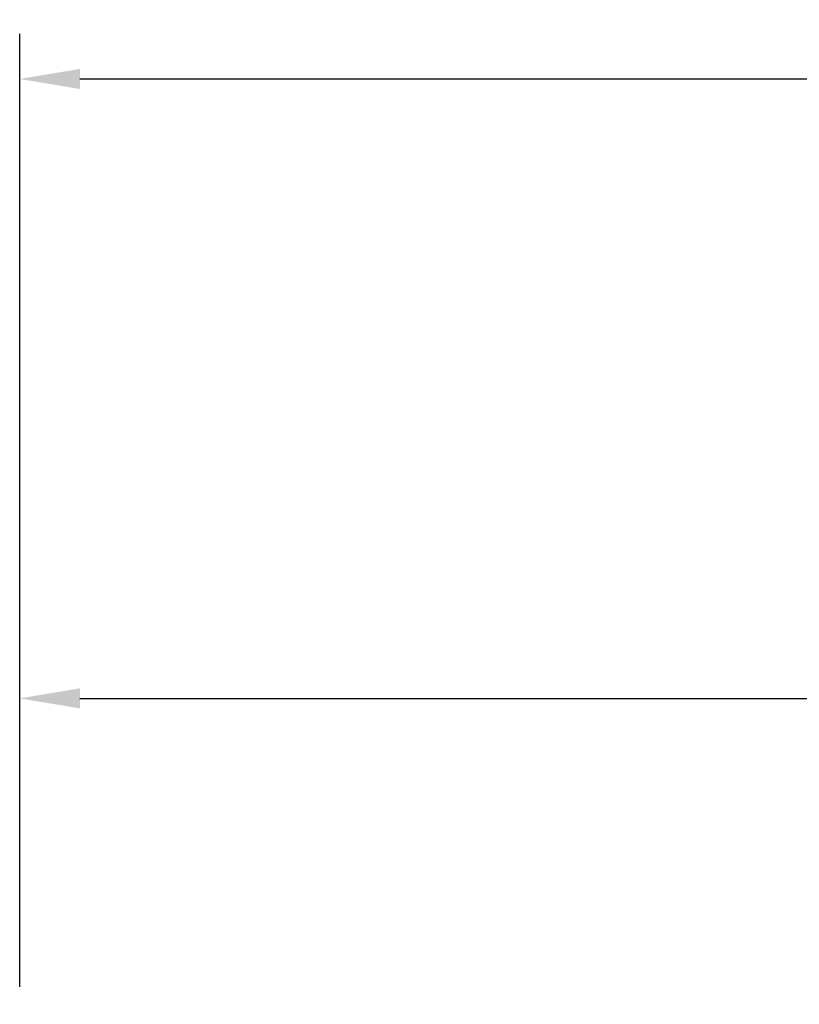
# Model space of a CAD drawing. Units: inches. Extents: x -59 to 502, y -260 to 136.
# Tile 4 of 8: x 25 to 77, y 66 to 131. Entities that reach past the tile are written whole.
import ezdxf

# ---------------------------------------------------------------- set-up
doc = ezdxf.new("R2010")
doc.units = ezdxf.units.IN
doc.header["$MEASUREMENT"] = 0
doc.layers.add('A-ANNO-DIMS', color=2, linetype='Continuous', lineweight=18)
doc.styles.get("Standard").update_dxf_attribs({"font": 'arial.ttf'})
doc.dimstyles.get("Standard").update_dxf_attribs({"dimtxt": 6, "dimasz": 4, "dimexe": 3, "dimexo": 3, "dimgap": 0.09, "dimtad": 0, "dimtih": 1, "dimtoh": 1, "dimdec": 1, "dimzin": 0, "dimdsep": 46, "dimlunit": 3, "dimtxsty": 'Standard', "dimcen": 0.09, "dimadec": 0, "dimazin": 0, "dimtfac": 1, "dimtdec": 1, "dimtofl": 0, "dimtmove": 0, "dimatfit": 3, "dimfxl": 1, "dimtolj": 1, "dimtzin": 0, "dimarcsym": 0})

# ---------------------------------------------------------------- blocks, each defined once
blk = doc.blocks.new('*D7')
at = {"layer": 'A-ANNO-DIMS', "color": 0, "lineweight": -2, "transparency": 16777216}
for p, q in [((25.459, 66.922), (25.459, 89.086)), ((421.459, 66.922), (421.459, 89.086)), ((29.459, 86.086), (218.28, 86.086)), ((417.459, 86.086), (228.638, 86.086))]:
    blk.add_line(p, q, dxfattribs=at)
at = {"layer": 'A-ANNO-DIMS', "color": 0, "transparency": 16777216}
for points in [[(29.459, 86.753), (29.459, 85.419), (25.459, 86.086)], [(417.459, 86.753), (417.459, 85.419), (421.459, 86.086)]]:
    blk.add_solid(points, dxfattribs=at)
at = {"layer": 'Defpoints', "color": 0, "transparency": 16777216}
for p in [(421.459, 86.086), (25.459, 63.922), (421.459, 63.922)]:
    blk.add_point(p, dxfattribs=at)
at = {"layer": 'A-ANNO-DIMS', "color": 0, "transparency": 16777216, "insert": (223.459, 86.086), "char_height": 6, "attachment_point": 5}
blk.add_mtext("\\A1;33'", dxfattribs=at)
blk = doc.blocks.new('*D57')
at = {"layer": 'A-ANNO-DIMS', "color": 0, "lineweight": -2, "transparency": 16777216}
for p, q in [((25.459, 66.922), (25.459, 130.246)), ((184.378, 66.922), (184.378, 130.246)), ((29.459, 127.246), (94.805, 127.246)), ((180.378, 127.246), (115.032, 127.246))]:
    blk.add_line(p, q, dxfattribs=at)
at = {"layer": 'A-ANNO-DIMS', "color": 0, "transparency": 16777216}
for points in [[(29.459, 127.913), (29.459, 126.58), (25.459, 127.246)], [(180.378, 127.913), (180.378, 126.58), (184.378, 127.246)]]:
    blk.add_solid(points, dxfattribs=at)
at = {"layer": 'Defpoints', "color": 0, "transparency": 16777216}
for p in [(184.378, 127.246), (25.459, 63.922), (184.378, 63.922)]:
    blk.add_point(p, dxfattribs=at)
at = {"layer": 'A-ANNO-DIMS', "color": 0, "transparency": 16777216, "insert": (104.919, 127.246), "char_height": 6, "attachment_point": 5}
blk.add_mtext('\\A1;13\'-3"', dxfattribs=at)

msp = doc.modelspace()

# ---------------------------------------------------------------- dimensions: what is measured, and where the dimension line sits
at = {"layer": 'A-ANNO-DIMS'}
for base, p2, override, picture, middle in [((184.378, 127.246), (184.378, 63.922), {"dimdec": 1, "dimlfac": 1, "dimrnd": 0, "dimzin": 1, "dimdsep": 46, "dimlunit": 4, "dimfrac": 2}, '*D57', (104.919, 127.246)), ((421.459, 86.086), (421.459, 63.922), {"dimclrd": 0, "dimclre": 0, "dimclrt": 0}, '*D7', (223.459, 86.086))]:
    dim = msp.add_linear_dim(base=base, p1=(25.459, 63.922), p2=p2, dimstyle='Standard', override=override, dxfattribs=at)
    dim.commit()
    dim.dimension.update_dxf_attribs({"geometry": picture, "text_midpoint": middle})

doc.saveas('drawing.dxf')
